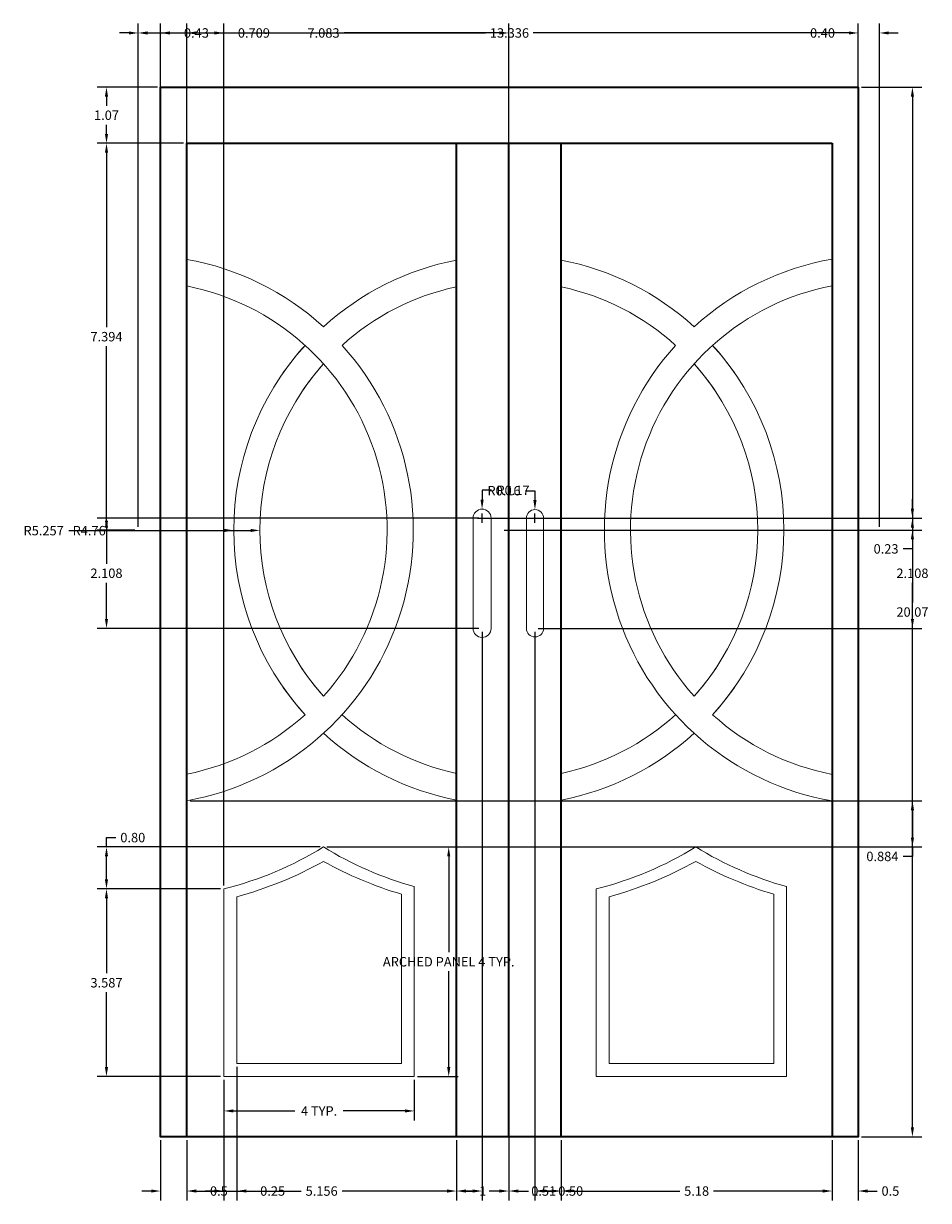
# Model space of a CAD drawing. Units: inches. Extents: x 13.4 to 30.7, y 29.2 to 51.7.
import ezdxf

# ---------------------------------------------------------------- set-up
doc = ezdxf.new("R2010")
doc.units = ezdxf.units.IN
doc.header["$MEASUREMENT"] = 0
for name, color, linetype, lineweight in [('A-ANNO-DIMS', 2, 'Continuous', 18), ('A-DOOR', 4, 'Continuous', 35), ('A-DOOR-HDWR', 6, 'Continuous', 18), ('A-DOOR-PANL', 3, 'Continuous', 18)]:
    doc.layers.add(name, color=color, linetype=linetype, lineweight=lineweight)
doc.styles.get("Standard").update_dxf_attribs({"font": 'arial.ttf'})
doc.dimstyles.get("Standard").update_dxf_attribs({"dimtxt": 0.18, "dimasz": 0.18, "dimexe": 0.18, "dimexo": 0.0625, "dimgap": 0.09, "dimtad": 0, "dimtih": 1, "dimtoh": 1, "dimdec": 4, "dimzin": 0, "dimdsep": 46, "dimtxsty": 'Standard', "dimcen": 0.09, "dimadec": 0, "dimazin": 0, "dimtfac": 1, "dimtdec": 4, "dimtofl": 0, "dimtmove": 0, "dimatfit": 3, "dimfxl": 1, "dimtolj": 1, "dimtzin": 0, "dimarcsym": 0})

# ---------------------------------------------------------------- blocks, each defined once
blk = doc.blocks.new('DOOR-PANEL-ARCH')
for points in [[(0, 3.587, 0.076922), (1.905, 4.388, 0.07036), (3.64, 3.632), (3.64, 0), (0, 0)], [(0.247, 3.438, 0.061893), (1.905, 4.113, 0.05583), (3.394, 3.486), (3.394, 0.246), (0.247, 0.246)]]:
    blk.add_lwpolyline(points, format="xyb", close=True)
blk = doc.blocks.new('*D2')
at = {"layer": 'A-ANNO-DIMS', "color": 0, "lineweight": -2, "transparency": 16777216}
for p, q in [((20.893, 35.948), (21.669, 35.948)), ((21.489, 35.768), (21.489, 33.937)), ((21.489, 31.74), (21.489, 33.571)), ((20.893, 31.56), (21.669, 31.56))]:
    blk.add_line(p, q, dxfattribs=at)
at = {"layer": 'A-ANNO-DIMS', "color": 0, "transparency": 16777216}
for points in [[(21.459, 35.768), (21.519, 35.768), (21.489, 35.948)], [(21.459, 31.74), (21.519, 31.74), (21.489, 31.56)]]:
    blk.add_solid(points, dxfattribs=at)
at = {"layer": 'Defpoints', "color": 0, "transparency": 16777216}
for p in [(20.831, 35.948), (21.489, 35.948), (20.831, 31.56)]:
    blk.add_point(p, dxfattribs=at)
at = {"layer": 'A-ANNO-DIMS', "color": 0, "transparency": 16777216, "insert": (21.489, 33.754), "char_height": 0.18, "attachment_point": 5}
blk.add_mtext('\\A1;ARCHED PANEL 4 TYP.', dxfattribs=at)
blk = doc.blocks.new('*D3')
at = {"layer": 'A-ANNO-DIMS', "color": 0, "lineweight": -2, "transparency": 16777216}
for p, q in [((17.191, 31.497), (17.191, 30.722)), ((20.831, 31.497), (20.831, 30.722)), ((17.371, 30.902), (18.549, 30.902)), ((20.651, 30.902), (19.473, 30.902))]:
    blk.add_line(p, q, dxfattribs=at)
at = {"layer": 'A-ANNO-DIMS', "color": 0, "transparency": 16777216}
for points in [[(17.371, 30.932), (17.371, 30.872), (17.191, 30.902)], [(20.651, 30.932), (20.651, 30.872), (20.831, 30.902)]]:
    blk.add_solid(points, dxfattribs=at)
at = {"layer": 'Defpoints', "color": 0, "transparency": 16777216}
for p in [(17.191, 31.56), (20.831, 31.56), (20.831, 30.902)]:
    blk.add_point(p, dxfattribs=at)
at = {"layer": 'A-ANNO-DIMS', "color": 0, "transparency": 16777216, "insert": (19.011, 30.902), "char_height": 0.18, "attachment_point": 5}
blk.add_mtext('\\A1;4 TYP.', dxfattribs=at)
blk = doc.blocks.new('*D4')
at = {"layer": 'A-ANNO-DIMS', "color": 0, "lineweight": -2, "transparency": 16777216}
for p, q in [((15.982, 50.538), (15.982, 51.69)), ((29.318, 50.538), (29.318, 51.69)), ((16.162, 51.51), (22.195, 51.51)), ((29.138, 51.51), (23.105, 51.51))]:
    blk.add_line(p, q, dxfattribs=at)
at = {"layer": 'A-ANNO-DIMS', "color": 0, "transparency": 16777216}
for points in [[(16.162, 51.54), (16.162, 51.48), (15.982, 51.51)], [(29.138, 51.54), (29.138, 51.48), (29.318, 51.51)]]:
    blk.add_solid(points, dxfattribs=at)
at = {"layer": 'Defpoints', "color": 0, "transparency": 16777216}
for p in [(29.318, 51.51), (15.982, 50.475), (29.318, 50.475)]:
    blk.add_point(p, dxfattribs=at)
at = {"layer": 'A-ANNO-DIMS', "color": 0, "transparency": 16777216, "insert": (22.65, 51.51), "char_height": 0.18, "attachment_point": 5}
blk.add_mtext('\\A1;13.336', dxfattribs=at)
blk = doc.blocks.new('*D5')
at = {"layer": 'A-ANNO-DIMS', "color": 0, "lineweight": -2, "transparency": 16777216}
for p, q in [((29.38, 50.475), (30.533, 50.475)), ((30.353, 50.295), (30.353, 40.622)), ((30.353, 30.586), (30.353, 40.259)), ((29.38, 30.406), (30.533, 30.406))]:
    blk.add_line(p, q, dxfattribs=at)
at = {"layer": 'A-ANNO-DIMS', "color": 0, "transparency": 16777216}
for points in [[(30.323, 50.295), (30.383, 50.295), (30.353, 50.475)], [(30.323, 30.586), (30.383, 30.586), (30.353, 30.406)]]:
    blk.add_solid(points, dxfattribs=at)
at = {"layer": 'Defpoints', "color": 0, "transparency": 16777216}
for p in [(29.318, 50.475), (30.353, 50.475), (29.318, 30.406)]:
    blk.add_point(p, dxfattribs=at)
at = {"layer": 'A-ANNO-DIMS', "color": 0, "transparency": 16777216, "insert": (30.353, 40.44), "char_height": 0.18, "attachment_point": 5}
blk.add_mtext('\\A1;20.07', dxfattribs=at)
blk = doc.blocks.new('*D6')
at = {"layer": 'A-ANNO-DIMS', "color": 0, "lineweight": -2, "transparency": 16777216}
for p, q in [((15.919, 50.475), (14.767, 50.475)), ((14.947, 50.295), (14.947, 50.12)), ((14.947, 49.581), (14.947, 49.756)), ((16.419, 49.401), (14.767, 49.401))]:
    blk.add_line(p, q, dxfattribs=at)
at = {"layer": 'A-ANNO-DIMS', "color": 0, "transparency": 16777216}
for points in [[(14.917, 50.295), (14.977, 50.295), (14.947, 50.475)], [(14.917, 49.581), (14.977, 49.581), (14.947, 49.401)]]:
    blk.add_solid(points, dxfattribs=at)
at = {"layer": 'Defpoints', "color": 0, "transparency": 16777216}
for p in [(14.947, 50.475), (15.982, 50.475), (16.482, 49.401)]:
    blk.add_point(p, dxfattribs=at)
at = {"layer": 'A-ANNO-DIMS', "color": 0, "transparency": 16777216, "insert": (14.947, 49.938), "char_height": 0.18, "attachment_point": 5}
blk.add_mtext('\\A1;1.07', dxfattribs=at)
blk = doc.blocks.new('*D7')
at = {"layer": 'A-ANNO-DIMS', "color": 0, "lineweight": -2, "transparency": 16777216}
for p, q in [((16.419, 49.401), (14.767, 49.401)), ((14.947, 49.221), (14.947, 45.886)), ((14.947, 42.187), (14.947, 45.522)), ((15.492, 42.007), (14.767, 42.007))]:
    blk.add_line(p, q, dxfattribs=at)
at = {"layer": 'A-ANNO-DIMS', "color": 0, "transparency": 16777216}
for points in [[(14.917, 49.221), (14.977, 49.221), (14.947, 49.401)], [(14.917, 42.187), (14.977, 42.187), (14.947, 42.007)]]:
    blk.add_solid(points, dxfattribs=at)
at = {"layer": 'Defpoints', "color": 0, "transparency": 16777216}
for p in [(14.947, 49.401), (16.482, 49.401), (15.555, 42.007)]:
    blk.add_point(p, dxfattribs=at)
at = {"layer": 'A-ANNO-DIMS', "color": 0, "transparency": 16777216, "insert": (14.947, 45.704), "char_height": 0.18, "attachment_point": 5}
blk.add_mtext('\\A1;7.394', dxfattribs=at)
blk = doc.blocks.new('*D8')
at = {"layer": 'A-ANNO-DIMS', "color": 0, "lineweight": -2, "transparency": 16777216}
for p, q in [((15.982, 30.343), (15.982, 29.191)), ((16.482, 30.343), (16.482, 29.191)), ((15.802, 29.371), (15.622, 29.371)), ((16.662, 29.371), (16.842, 29.371))]:
    blk.add_line(p, q, dxfattribs=at)
at = {"layer": 'A-ANNO-DIMS', "color": 0, "transparency": 16777216}
for points in [[(15.802, 29.401), (15.802, 29.341), (15.982, 29.371)], [(16.662, 29.401), (16.662, 29.341), (16.482, 29.371)]]:
    blk.add_solid(points, dxfattribs=at)
at = {"layer": 'Defpoints', "color": 0, "transparency": 16777216}
for p in [(15.982, 30.406), (16.482, 30.406), (16.482, 29.371)]:
    blk.add_point(p, dxfattribs=at)
at = {"layer": 'A-ANNO-DIMS', "color": 0, "transparency": 16777216, "insert": (17.096, 29.371), "char_height": 0.18, "attachment_point": 5}
blk.add_mtext('\\A1;0.5', dxfattribs=at)
blk = doc.blocks.new('*D9')
at = {"layer": 'A-ANNO-DIMS', "color": 0, "lineweight": -2, "transparency": 16777216}
for p, q in [((16.482, 30.343), (16.482, 29.191)), ((21.638, 30.343), (21.638, 29.191)), ((16.662, 29.371), (18.666, 29.371)), ((21.458, 29.371), (19.454, 29.371))]:
    blk.add_line(p, q, dxfattribs=at)
at = {"layer": 'A-ANNO-DIMS', "color": 0, "transparency": 16777216}
for points in [[(16.662, 29.401), (16.662, 29.341), (16.482, 29.371)], [(21.458, 29.401), (21.458, 29.341), (21.638, 29.371)]]:
    blk.add_solid(points, dxfattribs=at)
at = {"layer": 'Defpoints', "color": 0, "transparency": 16777216}
for p in [(16.482, 30.406), (21.638, 30.406), (21.638, 29.371)]:
    blk.add_point(p, dxfattribs=at)
at = {"layer": 'A-ANNO-DIMS', "color": 0, "transparency": 16777216, "insert": (19.06, 29.371), "char_height": 0.18, "attachment_point": 5}
blk.add_mtext('\\A1;5.156', dxfattribs=at)
blk = doc.blocks.new('*D10')
at = {"layer": 'A-ANNO-DIMS', "color": 0, "lineweight": -2, "transparency": 16777216}
for p, q in [((21.638, 30.343), (21.638, 29.191)), ((22.638, 30.343), (22.638, 29.191)), ((21.818, 29.371), (22.015, 29.371)), ((22.458, 29.371), (22.261, 29.371))]:
    blk.add_line(p, q, dxfattribs=at)
at = {"layer": 'A-ANNO-DIMS', "color": 0, "transparency": 16777216}
for points in [[(21.818, 29.401), (21.818, 29.341), (21.638, 29.371)], [(22.458, 29.401), (22.458, 29.341), (22.638, 29.371)]]:
    blk.add_solid(points, dxfattribs=at)
at = {"layer": 'Defpoints', "color": 0, "transparency": 16777216}
for p in [(21.638, 30.406), (22.638, 30.406), (22.638, 29.371)]:
    blk.add_point(p, dxfattribs=at)
at = {"layer": 'A-ANNO-DIMS', "color": 0, "transparency": 16777216, "insert": (22.138, 29.371), "char_height": 0.18, "attachment_point": 5}
blk.add_mtext('\\A1;1', dxfattribs=at)
blk = doc.blocks.new('*D11')
at = {"layer": 'A-ANNO-DIMS', "color": 0, "lineweight": -2, "transparency": 16777216}
for p, q in [((22.638, 30.343), (22.638, 29.191)), ((23.638, 30.343), (23.638, 29.191)), ((22.818, 29.371), (23.015, 29.371)), ((23.458, 29.371), (23.261, 29.371))]:
    blk.add_line(p, q, dxfattribs=at)
at = {"layer": 'A-ANNO-DIMS', "color": 0, "transparency": 16777216}
for points in [[(22.818, 29.401), (22.818, 29.341), (22.638, 29.371)], [(23.458, 29.401), (23.458, 29.341), (23.638, 29.371)]]:
    blk.add_solid(points, dxfattribs=at)
at = {"layer": 'Defpoints', "color": 0, "transparency": 16777216}
for p in [(22.638, 30.406), (23.638, 30.406), (23.638, 29.371)]:
    blk.add_point(p, dxfattribs=at)
at = {"layer": 'A-ANNO-DIMS', "color": 0, "transparency": 16777216, "insert": (23.138, 29.371), "char_height": 0.18, "attachment_point": 5}
blk.add_mtext('\\A1;1', dxfattribs=at)
blk = doc.blocks.new('*D12')
at = {"layer": 'A-ANNO-DIMS', "color": 0, "lineweight": -2, "transparency": 16777216}
for p, q in [((23.638, 30.343), (23.638, 29.191)), ((28.818, 30.343), (28.818, 29.191)), ((23.818, 29.371), (25.904, 29.371)), ((28.638, 29.371), (26.552, 29.371))]:
    blk.add_line(p, q, dxfattribs=at)
at = {"layer": 'A-ANNO-DIMS', "color": 0, "transparency": 16777216}
for points in [[(23.818, 29.401), (23.818, 29.341), (23.638, 29.371)], [(28.638, 29.401), (28.638, 29.341), (28.818, 29.371)]]:
    blk.add_solid(points, dxfattribs=at)
at = {"layer": 'Defpoints', "color": 0, "transparency": 16777216}
for p in [(23.638, 30.406), (28.818, 30.406), (28.818, 29.371)]:
    blk.add_point(p, dxfattribs=at)
at = {"layer": 'A-ANNO-DIMS', "color": 0, "transparency": 16777216, "insert": (26.228, 29.371), "char_height": 0.18, "attachment_point": 5}
blk.add_mtext('\\A1;5.18', dxfattribs=at)
blk = doc.blocks.new('*D13')
at = {"layer": 'A-ANNO-DIMS', "color": 0, "lineweight": -2, "transparency": 16777216}
for p, q in [((28.818, 30.343), (28.818, 29.191)), ((29.318, 30.343), (29.318, 29.191)), ((28.638, 29.371), (28.458, 29.371)), ((29.498, 29.371), (29.678, 29.371))]:
    blk.add_line(p, q, dxfattribs=at)
at = {"layer": 'A-ANNO-DIMS', "color": 0, "transparency": 16777216}
for points in [[(28.638, 29.401), (28.638, 29.341), (28.818, 29.371)], [(29.498, 29.401), (29.498, 29.341), (29.318, 29.371)]]:
    blk.add_solid(points, dxfattribs=at)
at = {"layer": 'Defpoints', "color": 0, "transparency": 16777216}
for p in [(28.818, 30.406), (29.318, 30.406), (29.318, 29.371)]:
    blk.add_point(p, dxfattribs=at)
at = {"layer": 'A-ANNO-DIMS', "color": 0, "transparency": 16777216, "insert": (29.932, 29.371), "char_height": 0.18, "attachment_point": 5}
blk.add_mtext('\\A1;0.5', dxfattribs=at)
blk = doc.blocks.new('*D14')
at = {"layer": 'A-ANNO-DIMS', "color": 0, "lineweight": -2, "transparency": 16777216}
for p, q in [((15.555, 42.07), (15.555, 51.69)), ((15.982, 30.468), (15.982, 51.69)), ((15.375, 51.51), (15.195, 51.51)), ((16.162, 51.51), (16.342, 51.51))]:
    blk.add_line(p, q, dxfattribs=at)
at = {"layer": 'A-ANNO-DIMS', "color": 0, "transparency": 16777216}
for points in [[(15.375, 51.54), (15.375, 51.48), (15.555, 51.51)], [(16.162, 51.54), (16.162, 51.48), (15.982, 51.51)]]:
    blk.add_solid(points, dxfattribs=at)
at = {"layer": 'Defpoints', "color": 0, "transparency": 16777216}
for p in [(15.982, 51.51), (15.555, 42.007), (15.982, 30.406)]:
    blk.add_point(p, dxfattribs=at)
at = {"layer": 'A-ANNO-DIMS', "color": 0, "transparency": 16777216, "insert": (16.666, 51.51), "char_height": 0.18, "attachment_point": 5}
blk.add_mtext('\\A1;0.43', dxfattribs=at)
blk = doc.blocks.new('*D15')
at = {"layer": 'A-ANNO-DIMS', "color": 0, "lineweight": -2, "transparency": 16777216}
for p, q in [((29.318, 30.468), (29.318, 51.69)), ((29.721, 42.07), (29.721, 51.69)), ((29.138, 51.51), (28.958, 51.51)), ((29.901, 51.51), (30.081, 51.51))]:
    blk.add_line(p, q, dxfattribs=at)
at = {"layer": 'A-ANNO-DIMS', "color": 0, "transparency": 16777216}
for points in [[(29.138, 51.54), (29.138, 51.48), (29.318, 51.51)], [(29.901, 51.54), (29.901, 51.48), (29.721, 51.51)]]:
    blk.add_solid(points, dxfattribs=at)
at = {"layer": 'Defpoints', "color": 0, "transparency": 16777216}
for p in [(29.318, 51.51), (29.721, 42.007), (29.318, 30.406)]:
    blk.add_point(p, dxfattribs=at)
at = {"layer": 'A-ANNO-DIMS', "color": 0, "transparency": 16777216, "insert": (28.634, 51.51), "char_height": 0.18, "attachment_point": 5}
blk.add_mtext('\\A1;0.40', dxfattribs=at)
blk = doc.blocks.new('*D16')
at = {"layer": 'A-ANNO-DIMS', "color": 0, "lineweight": -2, "transparency": 16777216}
for p, q in [((15.555, 42.07), (15.555, 51.69)), ((22.638, 42.07), (22.638, 51.69)), ((15.735, 51.51), (18.703, 51.51)), ((22.458, 51.51), (19.489, 51.51))]:
    blk.add_line(p, q, dxfattribs=at)
at = {"layer": 'A-ANNO-DIMS', "color": 0, "transparency": 16777216}
for points in [[(15.735, 51.54), (15.735, 51.48), (15.555, 51.51)], [(22.458, 51.54), (22.458, 51.48), (22.638, 51.51)]]:
    blk.add_solid(points, dxfattribs=at)
at = {"layer": 'Defpoints', "color": 0, "transparency": 16777216}
for p in [(22.638, 51.51), (15.555, 42.007), (22.638, 42.007)]:
    blk.add_point(p, dxfattribs=at)
at = {"layer": 'A-ANNO-DIMS', "color": 0, "transparency": 16777216, "insert": (19.096, 51.51), "char_height": 0.18, "attachment_point": 5}
blk.add_mtext('\\A1;7.083', dxfattribs=at)
blk = doc.blocks.new('*D17')
at = {"layer": 'A-ANNO-DIMS', "color": 0, "lineweight": -2, "transparency": 16777216}
for p, q in [((16.482, 36.895), (16.482, 51.69)), ((17.191, 35.209), (17.191, 51.69)), ((16.662, 51.51), (17.011, 51.51)), ((17.191, 51.51), (17.371, 51.51))]:
    blk.add_line(p, q, dxfattribs=at)
at = {"layer": 'A-ANNO-DIMS', "color": 0, "transparency": 16777216}
for points in [[(16.662, 51.54), (16.662, 51.48), (16.482, 51.51)], [(17.011, 51.54), (17.011, 51.48), (17.191, 51.51)]]:
    blk.add_solid(points, dxfattribs=at)
at = {"layer": 'Defpoints', "color": 0, "transparency": 16777216}
for p in [(17.191, 51.51), (16.482, 36.832), (17.191, 35.147)]:
    blk.add_point(p, dxfattribs=at)
at = {"layer": 'A-ANNO-DIMS', "color": 0, "transparency": 16777216, "insert": (17.765, 51.51), "char_height": 0.18, "attachment_point": 5}
blk.add_mtext('\\A1;0.709', dxfattribs=at)
blk = doc.blocks.new('*D18')
at = {"layer": 'A-ANNO-DIMS', "color": 0, "lineweight": -2, "transparency": 16777216}
for p, q in [((16.544, 36.832), (30.533, 36.832)), ((30.353, 36.652), (30.353, 36.128)), ((19.159, 35.948), (30.533, 35.948)), ((30.353, 35.948), (30.353, 35.768)), ((30.353, 35.768), (30.173, 35.768))]:
    blk.add_line(p, q, dxfattribs=at)
at = {"layer": 'A-ANNO-DIMS', "color": 0, "transparency": 16777216}
for points in [[(30.323, 36.652), (30.383, 36.652), (30.353, 36.832)], [(30.323, 36.128), (30.383, 36.128), (30.353, 35.948)]]:
    blk.add_solid(points, dxfattribs=at)
at = {"layer": 'Defpoints', "color": 0, "transparency": 16777216}
for p in [(16.482, 36.832), (19.096, 35.948), (30.353, 35.948)]:
    blk.add_point(p, dxfattribs=at)
at = {"layer": 'A-ANNO-DIMS', "color": 0, "transparency": 16777216, "insert": (29.779, 35.768), "char_height": 0.18, "attachment_point": 5}
blk.add_mtext('\\A1;0.884', dxfattribs=at)
blk = doc.blocks.new('*D19')
at = {"layer": 'A-ANNO-DIMS', "color": 0, "lineweight": -2, "transparency": 16777216}
for p, q in [((17.128, 35.147), (14.767, 35.147)), ((14.947, 34.967), (14.947, 33.535)), ((14.947, 31.74), (14.947, 33.171)), ((17.128, 31.56), (14.767, 31.56))]:
    blk.add_line(p, q, dxfattribs=at)
at = {"layer": 'A-ANNO-DIMS', "color": 0, "transparency": 16777216}
for points in [[(14.917, 34.967), (14.977, 34.967), (14.947, 35.147)], [(14.917, 31.74), (14.977, 31.74), (14.947, 31.56)]]:
    blk.add_solid(points, dxfattribs=at)
at = {"layer": 'Defpoints', "color": 0, "transparency": 16777216}
for p in [(14.947, 35.147), (17.191, 35.147), (17.191, 31.56)]:
    blk.add_point(p, dxfattribs=at)
at = {"layer": 'A-ANNO-DIMS', "color": 0, "transparency": 16777216, "insert": (14.947, 33.353), "char_height": 0.18, "attachment_point": 5}
blk.add_mtext('\\A1;3.587', dxfattribs=at)
blk = doc.blocks.new('*D20')
at = {"layer": 'A-ANNO-DIMS', "color": 0, "lineweight": -2, "transparency": 16777216}
for p, q in [((14.947, 35.948), (14.947, 36.128)), ((14.947, 36.128), (15.127, 36.128)), ((19.034, 35.948), (14.767, 35.948)), ((14.947, 35.327), (14.947, 35.768)), ((17.128, 35.147), (14.767, 35.147))]:
    blk.add_line(p, q, dxfattribs=at)
at = {"layer": 'A-ANNO-DIMS', "color": 0, "transparency": 16777216}
for points in [[(14.917, 35.768), (14.977, 35.768), (14.947, 35.948)], [(14.917, 35.327), (14.977, 35.327), (14.947, 35.147)]]:
    blk.add_solid(points, dxfattribs=at)
at = {"layer": 'Defpoints', "color": 0, "transparency": 16777216}
for p in [(14.947, 35.948), (19.096, 35.948), (17.191, 35.147)]:
    blk.add_point(p, dxfattribs=at)
at = {"layer": 'A-ANNO-DIMS', "color": 0, "transparency": 16777216, "insert": (15.45, 36.128), "char_height": 0.18, "attachment_point": 5}
blk.add_mtext('\\A1;0.80', dxfattribs=at)
blk = doc.blocks.new('*D21')
at = {"layer": 'A-ANNO-DIMS', "color": 0, "lineweight": -2, "transparency": 16777216}
for p, q in [((17.438, 31.744), (17.438, 29.191)), ((17.191, 31.497), (17.191, 29.191)), ((17.011, 29.371), (16.831, 29.371)), ((17.618, 29.371), (17.798, 29.371))]:
    blk.add_line(p, q, dxfattribs=at)
at = {"layer": 'A-ANNO-DIMS', "color": 0, "transparency": 16777216}
for points in [[(17.011, 29.401), (17.011, 29.341), (17.191, 29.371)], [(17.618, 29.401), (17.618, 29.341), (17.438, 29.371)]]:
    blk.add_solid(points, dxfattribs=at)
at = {"layer": 'Defpoints', "color": 0, "transparency": 16777216}
for p in [(17.438, 31.806), (17.191, 31.56), (17.438, 29.371)]:
    blk.add_point(p, dxfattribs=at)
at = {"layer": 'A-ANNO-DIMS', "color": 0, "transparency": 16777216, "insert": (18.123, 29.371), "char_height": 0.18, "attachment_point": 5}
blk.add_mtext('\\A1;0.25', dxfattribs=at)
blk = doc.blocks.new('*D22')
at = {"layer": 'A-ANNO-DIMS', "color": 0, "lineweight": -2, "transparency": 16777216}
for p, q in [((22.064, 42.235), (14.767, 42.235)), ((14.947, 42.055), (14.947, 41.363)), ((14.947, 40.307), (14.947, 40.999)), ((22.064, 40.127), (14.767, 40.127))]:
    blk.add_line(p, q, dxfattribs=at)
at = {"layer": 'A-ANNO-DIMS', "color": 0, "transparency": 16777216}
for points in [[(14.917, 42.055), (14.977, 42.055), (14.947, 42.235)], [(14.917, 40.307), (14.977, 40.307), (14.947, 40.127)]]:
    blk.add_solid(points, dxfattribs=at)
at = {"layer": 'Defpoints', "color": 0, "transparency": 16777216}
for p in [(22.127, 42.235), (14.947, 40.127), (22.127, 40.127)]:
    blk.add_point(p, dxfattribs=at)
at = {"layer": 'A-ANNO-DIMS', "color": 0, "transparency": 16777216, "insert": (14.947, 41.181), "char_height": 0.18, "attachment_point": 5}
blk.add_mtext('\\A1;2.108', dxfattribs=at)
blk = doc.blocks.new('*D23')
at = {"layer": 'A-ANNO-DIMS', "color": 0, "lineweight": -2, "transparency": 16777216}
for p, q in [((23.2, 42.235), (30.533, 42.235)), ((30.353, 42.055), (30.353, 41.363)), ((30.353, 40.307), (30.353, 40.999)), ((23.2, 40.127), (30.533, 40.127))]:
    blk.add_line(p, q, dxfattribs=at)
at = {"layer": 'A-ANNO-DIMS', "color": 0, "transparency": 16777216}
for points in [[(30.323, 42.055), (30.383, 42.055), (30.353, 42.235)], [(30.323, 40.307), (30.383, 40.307), (30.353, 40.127)]]:
    blk.add_solid(points, dxfattribs=at)
at = {"layer": 'Defpoints', "color": 0, "transparency": 16777216}
for p in [(23.137, 42.235), (23.137, 40.127), (30.353, 40.127)]:
    blk.add_point(p, dxfattribs=at)
at = {"layer": 'A-ANNO-DIMS', "color": 0, "transparency": 16777216, "insert": (30.353, 41.181), "char_height": 0.18, "attachment_point": 5}
blk.add_mtext('\\A1;2.108', dxfattribs=at)
blk = doc.blocks.new('*D24')
at = {"layer": 'A-ANNO-DIMS', "color": 0, "lineweight": -2, "transparency": 16777216}
for p, q in [((22.638, 41.945), (22.638, 29.191)), ((22.127, 40.064), (22.127, 29.191)), ((21.947, 29.371), (21.767, 29.371)), ((22.818, 29.371), (22.998, 29.371))]:
    blk.add_line(p, q, dxfattribs=at)
at = {"layer": 'A-ANNO-DIMS', "color": 0, "transparency": 16777216}
for points in [[(21.947, 29.401), (21.947, 29.341), (22.127, 29.371)], [(22.818, 29.401), (22.818, 29.341), (22.638, 29.371)]]:
    blk.add_solid(points, dxfattribs=at)
at = {"layer": 'Defpoints', "color": 0, "transparency": 16777216}
for p in [(22.638, 42.007), (22.127, 40.127), (22.638, 29.371)]:
    blk.add_point(p, dxfattribs=at)
at = {"layer": 'A-ANNO-DIMS', "color": 0, "transparency": 16777216, "insert": (23.304, 29.371), "char_height": 0.18, "attachment_point": 5}
blk.add_mtext('\\A1;0.51', dxfattribs=at)
blk = doc.blocks.new('*D25')
at = {"layer": 'A-ANNO-DIMS', "color": 0, "lineweight": -2, "transparency": 16777216}
for p, q in [((22.638, 41.945), (22.638, 29.191)), ((23.137, 40.064), (23.137, 29.191)), ((22.458, 29.371), (22.278, 29.371)), ((23.317, 29.371), (23.497, 29.371))]:
    blk.add_line(p, q, dxfattribs=at)
at = {"layer": 'A-ANNO-DIMS', "color": 0, "transparency": 16777216}
for points in [[(22.458, 29.401), (22.458, 29.341), (22.638, 29.371)], [(23.317, 29.401), (23.317, 29.341), (23.137, 29.371)]]:
    blk.add_solid(points, dxfattribs=at)
at = {"layer": 'Defpoints', "color": 0, "transparency": 16777216}
for p in [(22.638, 42.007), (23.137, 40.127), (23.137, 29.371)]:
    blk.add_point(p, dxfattribs=at)
at = {"layer": 'A-ANNO-DIMS', "color": 0, "transparency": 16777216, "insert": (23.821, 29.371), "char_height": 0.18, "attachment_point": 5}
blk.add_mtext('\\A1;0.50', dxfattribs=at)
blk = doc.blocks.new('*D26')
at = {"layer": 'A-ANNO-DIMS', "color": 0, "lineweight": -2, "transparency": 16777216}
for p, q in [((30.353, 42.415), (30.353, 42.595)), ((22.189, 42.235), (30.533, 42.235)), ((22.7, 42.007), (30.533, 42.007)), ((30.353, 41.647), (30.173, 41.647)), ((30.353, 41.827), (30.353, 41.647))]:
    blk.add_line(p, q, dxfattribs=at)
at = {"layer": 'A-ANNO-DIMS', "color": 0, "transparency": 16777216}
for points in [[(30.323, 42.415), (30.383, 42.415), (30.353, 42.235)], [(30.323, 41.827), (30.383, 41.827), (30.353, 42.007)]]:
    blk.add_solid(points, dxfattribs=at)
at = {"layer": 'Defpoints', "color": 0, "transparency": 16777216}
for p in [(22.127, 42.235), (22.638, 42.007), (30.353, 42.007)]:
    blk.add_point(p, dxfattribs=at)
at = {"layer": 'A-ANNO-DIMS', "color": 0, "transparency": 16777216, "insert": (29.849, 41.647), "char_height": 0.18, "attachment_point": 5}
blk.add_mtext('\\A1;0.23', dxfattribs=at)
blk = doc.blocks.new('*D27')
at = {"layer": 'A-ANNO-DIMS', "color": 0, "lineweight": -2, "transparency": 16777216}
for p, q in [((22.638, 41.917), (22.638, 42.097)), ((14.226, 41.996), (17.2, 42)), ((22.548, 42.007), (22.728, 42.007))]:
    blk.add_line(p, q, dxfattribs=at)
at = {"layer": 'A-ANNO-DIMS', "color": 0, "transparency": 16777216}
blk.add_solid([(17.2, 42.03), (17.201, 41.97), (17.38, 42)], dxfattribs=at)
at = {"layer": 'Defpoints', "color": 0, "transparency": 16777216}
for p in [(17.38, 42), (22.638, 42.007)]:
    blk.add_point(p, dxfattribs=at)
at = {"layer": 'A-ANNO-DIMS', "color": 0, "transparency": 16777216, "insert": (13.746, 41.996), "char_height": 0.18, "attachment_point": 5}
blk.add_mtext('\\A1;R5.257', dxfattribs=at)
blk = doc.blocks.new('*D28')
at = {"layer": 'A-ANNO-DIMS', "color": 0, "lineweight": -2, "transparency": 16777216}
for p, q in [((22.638, 41.917), (22.638, 42.097)), ((15.026, 41.996), (17.7, 42)), ((22.548, 42.007), (22.728, 42.007))]:
    blk.add_line(p, q, dxfattribs=at)
at = {"layer": 'A-ANNO-DIMS', "color": 0, "transparency": 16777216}
blk.add_solid([(17.7, 42.03), (17.701, 41.97), (17.88, 42)], dxfattribs=at)
at = {"layer": 'Defpoints', "color": 0, "transparency": 16777216}
for p in [(17.88, 42), (22.638, 42.007)]:
    blk.add_point(p, dxfattribs=at)
at = {"layer": 'A-ANNO-DIMS', "color": 0, "transparency": 16777216, "insert": (14.616, 41.996), "char_height": 0.18, "attachment_point": 5}
blk.add_mtext('\\A1;R4.76', dxfattribs=at)
blk = doc.blocks.new('*D29')
at = {"layer": 'A-ANNO-DIMS', "color": 0, "lineweight": -2, "transparency": 16777216}
for p, q in [((22.128, 42.767), (22.127, 42.587)), ((22.308, 42.767), (22.128, 42.767)), ((22.127, 42.145), (22.127, 42.325)), ((22.037, 42.235), (22.217, 42.235))]:
    blk.add_line(p, q, dxfattribs=at)
at = {"layer": 'A-ANNO-DIMS', "color": 0, "transparency": 16777216}
blk.add_solid([(22.097, 42.587), (22.157, 42.587), (22.127, 42.407)], dxfattribs=at)
at = {"layer": 'Defpoints', "color": 0, "transparency": 16777216}
for p in [(22.127, 42.407), (22.127, 42.235)]:
    blk.add_point(p, dxfattribs=at)
at = {"layer": 'A-ANNO-DIMS', "color": 0, "transparency": 16777216, "insert": (22.718, 42.767), "char_height": 0.18, "attachment_point": 5}
blk.add_mtext('\\A1;R0.17', dxfattribs=at)
blk = doc.blocks.new('*D30')
at = {"layer": 'A-ANNO-DIMS', "color": 0, "lineweight": -2, "transparency": 16777216}
for p, q in [((22.956, 42.759), (23.136, 42.759)), ((23.136, 42.759), (23.137, 42.579)), ((23.137, 42.145), (23.137, 42.325)), ((23.047, 42.235), (23.227, 42.235))]:
    blk.add_line(p, q, dxfattribs=at)
at = {"layer": 'A-ANNO-DIMS', "color": 0, "transparency": 16777216}
blk.add_solid([(23.167, 42.579), (23.107, 42.579), (23.137, 42.399)], dxfattribs=at)
at = {"layer": 'Defpoints', "color": 0, "transparency": 16777216}
for p in [(23.137, 42.399), (23.137, 42.235)]:
    blk.add_point(p, dxfattribs=at)
at = {"layer": 'A-ANNO-DIMS', "color": 0, "transparency": 16777216, "insert": (22.546, 42.759), "char_height": 0.18, "attachment_point": 5}
blk.add_mtext('\\A1;R0.16', dxfattribs=at)

msp = doc.modelspace()

# ---------------------------------------------------------------- linework, layer by layer
at = {"layer": 'A-DOOR'}
for p, q in [((16.4819, 49.4009), (28.8176, 49.4009)), ((21.638, 30.4057), (21.638, 49.4009)), ((22.638, 30.4057), (22.638, 49.4009)), ((23.638, 30.4057), (23.638, 49.4009))]:
    msp.add_line(p, q, dxfattribs=at)
msp.add_lwpolyline([(15.9819, 50.4753), (29.3176, 50.4753), (29.3176, 30.4057), (15.9819, 30.4057)], close=True, dxfattribs=at)
for points in [[(16.4819, 30.4057), (16.4819, 49.4009)], [(28.8176, 49.4009), (28.8176, 30.4057)]]:
    msp.add_lwpolyline(points, dxfattribs=at)
at = {"layer": 'A-DOOR-HDWR'}
for p, q in [((21.955, 42.235), (21.955, 40.127)), ((22.2984, 42.235), (22.2984, 40.127)), ((22.9736, 42.235), (22.9736, 40.127)), ((23.301, 42.235), (23.301, 40.127))]:
    msp.add_line(p, q, dxfattribs=at)
for centre, radius, start, end in [((22.1267, 42.235), 0.1717, 0, 180), ((23.1373, 42.235), 0.1637, 0, 180), ((22.1267, 40.127), 0.1717, 180, 0), ((23.1373, 40.127), 0.1637, 180, 0)]:
    msp.add_arc(centre, radius, start, end, dxfattribs=at)
at = {"layer": 'A-DOOR-PANL'}
for centre, radius, start, end in [((15.5545, 42.0073), 5.2575, 47.65036, 79.83986), ((22.638, 42.0073), 5.2575, 100.96476, 132.34964), ((22.638, 42.0073), 5.2575, 100.96476, 132.34964), ((22.638, 42.0073), 5.2575, 47.65036, 79.03524), ((22.638, 42.0073), 5.2575, 47.65036, 79.03524), ((29.7214, 42.0073), 5.2575, 99.89847, 132.34964), ((15.5545, 42.0073), 4.7575, 318.11209, 78.75882), ((22.638, 42.0073), 4.7575, 102.1338, 132.0791), ((22.638, 42.0073), 4.7575, 102.1338, 132.0791), ((22.638, 42.0073), 4.7575, 47.9209, 77.8662), ((22.638, 42.0073), 4.7575, 47.9209, 77.8662), ((29.7214, 42.0073), 4.7575, 100.951, 221.88791), ((15.5545, 42.0073), 5.2575, 280.16014, 42.19324), ((22.638, 42.0073), 5.2575, 137.80676, 222.19324), ((22.638, 42.0073), 5.2575, 137.80676, 145.08119), ((29.7214, 42.0073), 5.2575, 137.80676, 260.10153), ((22.638, 42.0073), 5.2575, 34.91881, 42.19324), ((22.638, 42.0073), 5.2575, 317.80676, 42.19324), ((22.638, 42.0073), 4.7575, 138.11209, 221.88791), ((22.638, 42.0073), 4.7575, 138.11209, 146.28861), ((22.638, 42.0073), 4.7575, 33.71139, 41.88791), ((22.638, 42.0073), 4.7575, 318.11209, 41.88791), ((22.638, 42.0073), 4.7575, 213.71139, 221.88791), ((22.638, 42.0073), 4.7575, 318.11209, 326.28861), ((22.638, 42.0073), 5.2575, 214.91881, 222.19324), ((22.638, 42.0073), 5.2575, 317.80676, 325.08119), ((15.5545, 42.0073), 4.7575, 281.24118, 312.0791), ((22.638, 42.0073), 4.7575, 227.9209, 257.8662), ((22.638, 42.0073), 4.7575, 227.9209, 257.8662), ((22.638, 42.0073), 4.7575, 282.1338, 312.0791), ((22.638, 42.0073), 4.7575, 282.1338, 312.0791), ((29.7214, 42.0073), 4.7575, 227.9209, 259.049), ((22.638, 42.0073), 5.2575, 227.65036, 259.03524), ((22.638, 42.0073), 5.2575, 227.65036, 259.03524), ((22.638, 42.0073), 5.2575, 280.96476, 312.34964), ((22.638, 42.0073), 5.2575, 280.96476, 312.34964)]:
    msp.add_arc(centre, radius, start, end, dxfattribs=at)

# ---------------------------------------------------------------- block references
for p in [(17.191, 31.56), (24.3066, 31.56)]:
    msp.add_blockref('DOOR-PANEL-ARCH', p, dxfattribs=at)

# ---------------------------------------------------------------- dimensions: what is measured, and where the dimension line sits
at = {"layer": 'A-ANNO-DIMS'}
for base, p1, p2, override, picture, middle in [((15.9819, 51.5103), (15.5545, 42.0073), (15.9819, 30.4057), {"dimdec": 2, "dimlfac": 1, "dimrnd": 0, "dimzin": 0, "dimdsep": 46, "dimlunit": 2}, '*D14', (16.6657, 51.5103)), ((22.63795, 51.5103), (15.55452, 42.00726), (22.63795, 42.00726), {"dimdec": 3, "dimlfac": 1, "dimrnd": 0, "dimzin": 0, "dimdsep": 46, "dimlunit": 2}, '*D16', (19.09624, 51.5103)), ((29.3176, 51.5103), (15.9819, 50.4753), (29.3176, 50.4753), {"dimdec": 3, "dimlfac": 1, "dimrnd": 0, "dimzin": 0, "dimdsep": 46, "dimlunit": 2}, '*D4', (22.6498, 51.5103)), ((17.1909, 51.5103), (16.4819, 36.8322), (17.1909, 35.1468), {"dimdec": 3, "dimlfac": 1, "dimrnd": 0, "dimzin": 0, "dimdsep": 46, "dimlunit": 2}, '*D17', (17.7648, 51.5103)), ((29.3176, 51.5103), (29.7214, 42.0073), (29.3176, 30.4057), {"dimdec": 2, "dimlfac": 1, "dimrnd": 0, "dimzin": 0, "dimdsep": 46, "dimlunit": 2}, '*D15', (28.6341, 51.5103)), ((22.638, 29.3707), (22.1267, 40.127), (22.638, 42.0073), {"dimdec": 2, "dimlfac": 1, "dimrnd": 0, "dimzin": 0, "dimdsep": 46, "dimlunit": 2}, '*D24', (23.3044, 29.3707)), ((23.1373, 29.3707), (22.638, 42.0073), (23.1373, 40.127), {"dimdec": 2, "dimlfac": 1, "dimrnd": 0, "dimzin": 0, "dimdsep": 46, "dimlunit": 2}, '*D25', (23.8208, 29.3707)), ((17.4382, 29.3707), (17.1909, 31.5598), (17.4382, 31.8061), {"dimdec": 2, "dimlfac": 1, "dimrnd": 0, "dimzin": 0, "dimdsep": 46, "dimlunit": 2}, '*D21', (18.1226, 29.3707)), ((16.4819, 29.3707), (15.9819, 30.4057), (16.4819, 30.4057), {"dimdec": 1, "dimlfac": 1, "dimrnd": 0, "dimzin": 0, "dimdsep": 46, "dimlunit": 2}, '*D8', (17.0965, 29.3707)), ((21.638, 29.3707), (16.4819, 30.4057), (21.638, 30.4057), {"dimdec": 3, "dimlfac": 1, "dimrnd": 0, "dimzin": 0, "dimdsep": 46, "dimlunit": 2}, '*D9', (19.0599, 29.3707)), ((22.638, 29.3707), (21.638, 30.4057), (22.638, 30.4057), {"dimdec": 0, "dimlfac": 1, "dimrnd": 0, "dimzin": 0, "dimdsep": 46, "dimlunit": 2}, '*D10', (22.138, 29.3707)), ((23.638, 29.3707), (22.638, 30.4057), (23.638, 30.4057), {"dimdec": 0, "dimlfac": 1, "dimrnd": 0, "dimzin": 0, "dimdsep": 46, "dimlunit": 2}, '*D11', (23.138, 29.3707)), ((28.8176, 29.3707), (23.638, 30.4057), (28.8176, 30.4057), {"dimdec": 2, "dimlfac": 1, "dimrnd": 0, "dimzin": 0, "dimdsep": 46, "dimlunit": 2}, '*D12', (26.2278, 29.3707)), ((29.3176, 29.3707), (28.8176, 30.4057), (29.3176, 30.4057), {"dimdec": 1, "dimlfac": 1, "dimrnd": 0, "dimzin": 0, "dimdsep": 46, "dimlunit": 2}, '*D13', (29.9321, 29.3707))]:
    dim = msp.add_linear_dim(base=base, p1=p1, p2=p2, dimstyle='Standard', override=override, dxfattribs=at)
    dim.commit()
    dim.dimension.update_dxf_attribs({"geometry": picture, "text_midpoint": middle})
for base, p1, p2, override, picture, middle in [((14.9469, 50.4753), (16.4819, 49.4009), (15.9819, 50.4753), {"dimdec": 2, "dimlfac": 1, "dimrnd": 0, "dimzin": 0, "dimdsep": 46, "dimlunit": 2}, '*D6', (14.9469, 49.9381)), ((30.3526, 50.4753), (29.3176, 30.4057), (29.3176, 50.4753), {"dimdec": 2, "dimlfac": 1, "dimrnd": 0, "dimzin": 0, "dimdsep": 46, "dimlunit": 2}, '*D5', (30.3526, 40.4405)), ((14.9469, 49.4009), (15.5545, 42.0073), (16.4819, 49.4009), {"dimdec": 3, "dimlfac": 1, "dimrnd": 0, "dimzin": 0, "dimdsep": 46, "dimlunit": 2}, '*D7', (14.9469, 45.7041)), ((30.3526, 42.0073), (22.1267, 42.235), (22.638, 42.0073), {"dimdec": 2, "dimlfac": 1, "dimrnd": 0, "dimzin": 0, "dimdsep": 46, "dimlunit": 2}, '*D26', (29.8488, 41.6473)), ((14.9469, 40.127), (22.1267, 42.235), (22.1267, 40.127), {"dimdec": 3, "dimlfac": 1, "dimrnd": 0, "dimzin": 0, "dimdsep": 46, "dimlunit": 2}, '*D22', (14.9469, 41.181)), ((30.3526, 40.127), (23.1373, 42.235), (23.1373, 40.127), {"dimdec": 3, "dimlfac": 1, "dimrnd": 0, "dimzin": 0, "dimdsep": 46, "dimlunit": 2}, '*D23', (30.3526, 41.181)), ((30.3526, 35.9481), (16.4819, 36.8322), (19.0962, 35.9481), {"dimdec": 3, "dimlfac": 1, "dimrnd": 0, "dimzin": 0, "dimdsep": 46, "dimlunit": 2}, '*D18', (29.7793, 35.7681)), ((14.9469, 35.9481), (17.1909, 35.1468), (19.0962, 35.9481), {"dimdec": 2, "dimlfac": 1, "dimrnd": 0, "dimzin": 0, "dimdsep": 46, "dimlunit": 2}, '*D20', (15.4504, 36.1281)), ((14.9469, 35.1468), (17.1909, 31.5598), (17.1909, 35.1468), {"dimdec": 3, "dimlfac": 1, "dimrnd": 0, "dimzin": 0, "dimdsep": 46, "dimlunit": 2}, '*D19', (14.9469, 33.3533))]:
    dim = msp.add_linear_dim(base=base, p1=p1, p2=p2, angle=90, dimstyle='Standard', override=override, dxfattribs=at)
    dim.commit()
    dim.dimension.update_dxf_attribs({"geometry": picture, "text_midpoint": middle})
for center, mpoint, picture, middle in [((22.1267, 42.235), (22.127, 42.4067), '*D29', (22.7176, 42.7667)), ((23.1373, 42.235), (23.137, 42.3987), '*D30', (22.5465, 42.7587))]:
    dim = msp.add_radius_dim(center=center, mpoint=mpoint, dimstyle='Standard', override={"dimdec": 2, "dimlfac": 1, "dimrnd": 0, "dimzin": 0, "dimdsep": 46, "dimlunit": 2}, dxfattribs=at)
    dim.commit()
    dim.dimension.update_dxf_attribs({"geometry": picture, "text_midpoint": middle})
for center, mpoint, override, picture, middle in [((22.63795, 42.00726), (17.38048, 42), {"dimdec": 3, "dimlfac": 1, "dimrnd": 0, "dimzin": 0, "dimdsep": 46, "dimlunit": 2}, '*D27', (14.226, 41.99565)), ((22.638, 42.0073), (17.8805, 42), {"dimdec": 2, "dimlfac": 1, "dimrnd": 0, "dimzin": 0, "dimdsep": 46, "dimlunit": 2}, '*D28', (15.026, 41.9956))]:
    dim = msp.add_radius_dim(center=center, mpoint=mpoint, dimstyle='Standard', override=override, dxfattribs=at)
    dim.commit()
    dim.dimension.update_dxf_attribs({"geometry": picture, "text_midpoint": middle, "dimtype": 164})
dim = msp.add_linear_dim(base=(21.4892, 35.9481), p1=(20.8309, 31.5598), p2=(20.8309, 35.9481), angle=90, text='ARCHED PANEL <> TYP.', dimstyle='Standard', override={"dimdec": 0, "dimrnd": 0, "dimzin": 0, "dimlunit": 2}, dxfattribs=at)
dim.commit()
dim.dimension.update_dxf_attribs({"geometry": '*D2', "text_midpoint": (21.4892, 33.754)})
dim = msp.add_linear_dim(base=(20.8309, 30.9015), p1=(17.1909, 31.5598), p2=(20.8309, 31.5598), text='<> TYP.', dimstyle='Standard', override={"dimdec": 0, "dimrnd": 0, "dimzin": 0, "dimlunit": 2}, dxfattribs=at)
dim.commit()
dim.dimension.update_dxf_attribs({"geometry": '*D3', "text_midpoint": (19.0109, 30.9015)})

doc.saveas('drawing.dxf')
